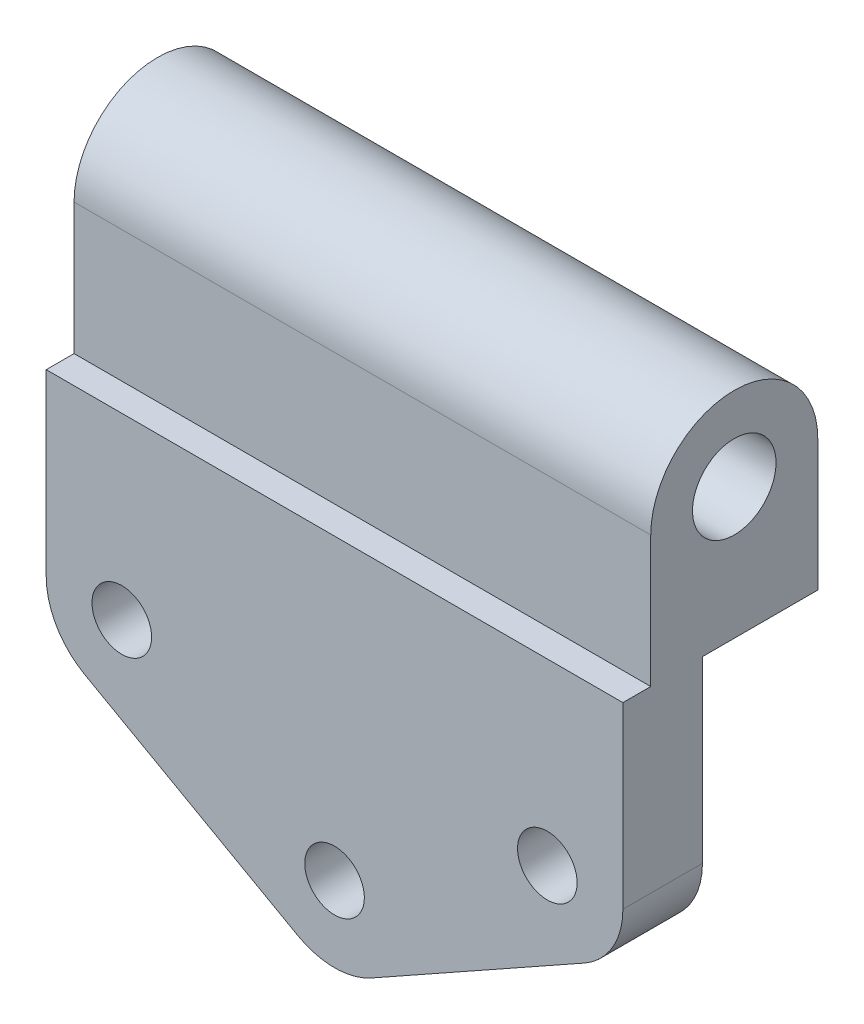
ISO-10303-21;
HEADER;
FILE_DESCRIPTION(('STEP AP214'),'2;1');
FILE_NAME('part.step','',(''),(''),'','','');
FILE_SCHEMA(('AUTOMOTIVE_DESIGN { 1 0 10303 214 1 1 1 1 }'));
ENDSEC;
DATA;
#1=APPLICATION_CONTEXT('core data for automotive mechanical design processes');
#2=APPLICATION_PROTOCOL_DEFINITION('international standard','automotive_design',2000,#1);
#3=PRODUCT_CONTEXT('',#1,'mechanical');
#4=PRODUCT('Part','Part','',(#3));
#5=PRODUCT_RELATED_PRODUCT_CATEGORY('part','',(#4));
#6=PRODUCT_DEFINITION_FORMATION('','',#4);
#7=PRODUCT_DEFINITION_CONTEXT('part definition',#1,'design');
#8=PRODUCT_DEFINITION('design','',#6,#7);
#9=PRODUCT_DEFINITION_SHAPE('','',#8);
#10=(LENGTH_UNIT() NAMED_UNIT(*) SI_UNIT(.MILLI.,.METRE.));
#11=(NAMED_UNIT(*) PLANE_ANGLE_UNIT() SI_UNIT($,.RADIAN.));
#12=(NAMED_UNIT(*) SI_UNIT($,.STERADIAN.) SOLID_ANGLE_UNIT());
#13=UNCERTAINTY_MEASURE_WITH_UNIT(LENGTH_MEASURE(1.E-05),#10,'distance_accuracy_value','');
#14=(GEOMETRIC_REPRESENTATION_CONTEXT(3) GLOBAL_UNCERTAINTY_ASSIGNED_CONTEXT((#13)) GLOBAL_UNIT_ASSIGNED_CONTEXT((#10,
#11,#12)) REPRESENTATION_CONTEXT('',''));
#15=CARTESIAN_POINT('',(0.,0.,0.));
#16=DIRECTION('',(0.,0.,1.));
#17=DIRECTION('',(1.,0.,0.));
#18=AXIS2_PLACEMENT_3D('',#15,#16,#17);
#19=CARTESIAN_POINT('',(-53.5,-16.9354535125797,20.));
#20=DIRECTION('',(0.,0.,1.));
#21=DIRECTION('',(1.,0.,0.));
#22=AXIS2_PLACEMENT_3D('',#19,#20,#21);
#23=PLANE('',#22);
#24=CARTESIAN_POINT('',(53.5,-16.9354535125797,20.));
#25=DIRECTION('',(0.,0.,1.));
#26=DIRECTION('',(1.,0.,0.));
#27=AXIS2_PLACEMENT_3D('',#24,#25,#26);
#28=CIRCLE('',#27,7.49226737139346);
#29=CARTESIAN_POINT('',(60.9922673713935,-16.9354535125797,20.));
#30=VERTEX_POINT('',#29);
#31=EDGE_CURVE('E198',#30,#30,#28,.T.);
#32=ORIENTED_EDGE('',*,*,#31,.F.);
#33=EDGE_LOOP('',(#32));
#34=FACE_BOUND('',#33,.T.);
#35=DIRECTION('',(0.,-1.,0.));
#36=VECTOR('',#35,1.);
#37=CARTESIAN_POINT('',(-72.5,28.0645464874203,20.));
#38=LINE('',#37,#36);
#39=CARTESIAN_POINT('',(-72.5,28.0645464874203,20.));
#40=VERTEX_POINT('',#39);
#41=CARTESIAN_POINT('',(-72.5,-16.9354535125796,20.));
#42=VERTEX_POINT('',#41);
#43=EDGE_CURVE('E158',#40,#42,#38,.T.);
#44=ORIENTED_EDGE('',*,*,#43,.T.);
#45=CARTESIAN_POINT('',(-53.5,-16.9354535125797,20.));
#46=DIRECTION('',(0.,0.,1.));
#47=DIRECTION('',(1.,0.,0.));
#48=AXIS2_PLACEMENT_3D('',#45,#46,#47);
#49=CIRCLE('',#48,19.);
#50=CARTESIAN_POINT('',(-62.792895002889,-33.5077829343984,20.));
#51=VERTEX_POINT('',#50);
#52=EDGE_CURVE('E97',#42,#51,#49,.T.);
#53=ORIENTED_EDGE('',*,*,#52,.T.);
#54=DIRECTION('',(0.872227864306251,-0.48909973699416,0.));
#55=VECTOR('',#54,1.);
#56=CARTESIAN_POINT('',(-62.792895002889,-33.5077829343984,20.));
#57=LINE('',#56,#55);
#58=CARTESIAN_POINT('',(-9.29289500288901,-63.5077829343984,20.));
#59=VERTEX_POINT('',#58);
#60=EDGE_CURVE('E173',#51,#59,#57,.T.);
#61=ORIENTED_EDGE('',*,*,#60,.T.);
#62=CARTESIAN_POINT('',(0.,-46.9354535125796,20.));
#63=DIRECTION('',(0.,0.,1.));
#64=DIRECTION('',(1.,0.,0.));
#65=AXIS2_PLACEMENT_3D('',#62,#63,#64);
#66=CIRCLE('',#65,19.);
#67=CARTESIAN_POINT('',(9.29289500288904,-63.5077829343984,20.));
#68=VERTEX_POINT('',#67);
#69=EDGE_CURVE('E186',#59,#68,#66,.T.);
#70=ORIENTED_EDGE('',*,*,#69,.T.);
#71=DIRECTION('',(0.872227864306251,0.489099736994159,0.));
#72=VECTOR('',#71,1.);
#73=CARTESIAN_POINT('',(62.792895002889,-33.5077829343985,20.));
#74=LINE('',#73,#72);
#75=CARTESIAN_POINT('',(62.792895002889,-33.5077829343985,20.));
#76=VERTEX_POINT('',#75);
#77=EDGE_CURVE('E117',#68,#76,#74,.T.);
#78=ORIENTED_EDGE('',*,*,#77,.T.);
#79=CARTESIAN_POINT('',(53.5,-16.9354535125797,20.));
#80=DIRECTION('',(0.,0.,1.));
#81=DIRECTION('',(1.,0.,0.));
#82=AXIS2_PLACEMENT_3D('',#79,#80,#81);
#83=CIRCLE('',#82,19.);
#84=CARTESIAN_POINT('',(72.5,-16.9354535125797,20.));
#85=VERTEX_POINT('',#84);
#86=EDGE_CURVE('E111',#76,#85,#83,.T.);
#87=ORIENTED_EDGE('',*,*,#86,.T.);
#88=DIRECTION('',(0.,1.,0.));
#89=VECTOR('',#88,1.);
#90=CARTESIAN_POINT('',(72.5,28.0645464874203,20.));
#91=LINE('',#90,#89);
#92=CARTESIAN_POINT('',(72.5,28.0645464874203,20.));
#93=VERTEX_POINT('',#92);
#94=EDGE_CURVE('E116',#85,#93,#91,.T.);
#95=ORIENTED_EDGE('',*,*,#94,.T.);
#96=DIRECTION('',(-1.,0.,0.));
#97=VECTOR('',#96,1.);
#98=CARTESIAN_POINT('',(-72.5,28.0645464874203,20.));
#99=LINE('',#98,#97);
#100=EDGE_CURVE('E65',#93,#40,#99,.T.);
#101=ORIENTED_EDGE('',*,*,#100,.T.);
#102=EDGE_LOOP('',(#44,#53,#61,#70,#78,#87,#95,#101));
#103=FACE_BOUND('',#102,.T.);
#104=CARTESIAN_POINT('',(0.,-46.9354535125796,20.));
#105=DIRECTION('',(0.,0.,1.));
#106=DIRECTION('',(1.,0.,0.));
#107=AXIS2_PLACEMENT_3D('',#104,#105,#106);
#108=CIRCLE('',#107,7.49226737139346);
#109=CARTESIAN_POINT('',(7.49226737139348,-46.9354535125796,20.));
#110=VERTEX_POINT('',#109);
#111=EDGE_CURVE('E145',#110,#110,#108,.T.);
#112=ORIENTED_EDGE('',*,*,#111,.F.);
#113=EDGE_LOOP('',(#112));
#114=FACE_BOUND('',#113,.T.);
#115=CARTESIAN_POINT('',(-53.5,-16.9354535125797,20.));
#116=DIRECTION('',(0.,0.,1.));
#117=DIRECTION('',(1.,0.,0.));
#118=AXIS2_PLACEMENT_3D('',#115,#116,#117);
#119=CIRCLE('',#118,7.49226737139346);
#120=CARTESIAN_POINT('',(-46.0077326286065,-16.9354535125797,20.));
#121=VERTEX_POINT('',#120);
#122=EDGE_CURVE('E205',#121,#121,#119,.T.);
#123=ORIENTED_EDGE('',*,*,#122,.F.);
#124=EDGE_LOOP('',(#123));
#125=FACE_BOUND('',#124,.T.);
#126=ADVANCED_FACE('F39',(#34,#103,#114,#125),#23,.T.);
#127=CARTESIAN_POINT('',(-53.5,-16.9354535125797,0.));
#128=DIRECTION('',(0.,0.,1.));
#129=DIRECTION('',(1.,0.,0.));
#130=AXIS2_PLACEMENT_3D('',#127,#128,#129);
#131=PLANE('',#130);
#132=DIRECTION('',(0.,-1.,0.));
#133=VECTOR('',#132,1.);
#134=CARTESIAN_POINT('',(-72.5,28.0645464874203,0.));
#135=LINE('',#134,#133);
#136=CARTESIAN_POINT('',(-72.5,28.0645464874203,0.));
#137=VERTEX_POINT('',#136);
#138=CARTESIAN_POINT('',(-72.5,-16.9354535125796,0.));
#139=VERTEX_POINT('',#138);
#140=EDGE_CURVE('E136',#137,#139,#135,.T.);
#141=ORIENTED_EDGE('',*,*,#140,.F.);
#142=DIRECTION('',(-1.,0.,0.));
#143=VECTOR('',#142,1.);
#144=CARTESIAN_POINT('',(-72.5,28.0645464874203,0.));
#145=LINE('',#144,#143);
#146=CARTESIAN_POINT('',(72.5,28.0645464874203,0.));
#147=VERTEX_POINT('',#146);
#148=EDGE_CURVE('E154',#147,#137,#145,.T.);
#149=ORIENTED_EDGE('',*,*,#148,.F.);
#150=DIRECTION('',(0.,1.,0.));
#151=VECTOR('',#150,1.);
#152=CARTESIAN_POINT('',(72.5,28.0645464874203,0.));
#153=LINE('',#152,#151);
#154=CARTESIAN_POINT('',(72.5,-16.9354535125797,0.));
#155=VERTEX_POINT('',#154);
#156=EDGE_CURVE('E153',#155,#147,#153,.T.);
#157=ORIENTED_EDGE('',*,*,#156,.F.);
#158=CARTESIAN_POINT('',(53.5,-16.9354535125797,0.));
#159=DIRECTION('',(0.,0.,1.));
#160=DIRECTION('',(1.,0.,0.));
#161=AXIS2_PLACEMENT_3D('',#158,#159,#160);
#162=CIRCLE('',#161,19.);
#163=CARTESIAN_POINT('',(62.792895002889,-33.5077829343985,0.));
#164=VERTEX_POINT('',#163);
#165=EDGE_CURVE('E93',#164,#155,#162,.T.);
#166=ORIENTED_EDGE('',*,*,#165,.F.);
#167=DIRECTION('',(0.872227864306251,0.489099736994159,0.));
#168=VECTOR('',#167,1.);
#169=CARTESIAN_POINT('',(62.792895002889,-33.5077829343985,0.));
#170=LINE('',#169,#168);
#171=CARTESIAN_POINT('',(9.29289500288904,-63.5077829343984,0.));
#172=VERTEX_POINT('',#171);
#173=EDGE_CURVE('E147',#172,#164,#170,.T.);
#174=ORIENTED_EDGE('',*,*,#173,.F.);
#175=CARTESIAN_POINT('',(0.,-46.9354535125796,0.));
#176=DIRECTION('',(0.,0.,1.));
#177=DIRECTION('',(1.,0.,0.));
#178=AXIS2_PLACEMENT_3D('',#175,#176,#177);
#179=CIRCLE('',#178,19.);
#180=CARTESIAN_POINT('',(-9.29289500288901,-63.5077829343984,0.));
#181=VERTEX_POINT('',#180);
#182=EDGE_CURVE('E146',#181,#172,#179,.T.);
#183=ORIENTED_EDGE('',*,*,#182,.F.);
#184=DIRECTION('',(0.872227864306251,-0.48909973699416,0.));
#185=VECTOR('',#184,1.);
#186=CARTESIAN_POINT('',(-62.792895002889,-33.5077829343984,0.));
#187=LINE('',#186,#185);
#188=CARTESIAN_POINT('',(-62.792895002889,-33.5077829343984,0.));
#189=VERTEX_POINT('',#188);
#190=EDGE_CURVE('E148',#189,#181,#187,.T.);
#191=ORIENTED_EDGE('',*,*,#190,.F.);
#192=CARTESIAN_POINT('',(-53.5,-16.9354535125797,0.));
#193=DIRECTION('',(0.,0.,1.));
#194=DIRECTION('',(1.,0.,0.));
#195=AXIS2_PLACEMENT_3D('',#192,#193,#194);
#196=CIRCLE('',#195,19.);
#197=EDGE_CURVE('E141',#139,#189,#196,.T.);
#198=ORIENTED_EDGE('',*,*,#197,.F.);
#199=EDGE_LOOP('',(#141,#149,#157,#166,#174,#183,#191,#198));
#200=FACE_BOUND('',#199,.T.);
#201=CARTESIAN_POINT('',(0.,-46.9354535125796,0.));
#202=DIRECTION('',(0.,0.,1.));
#203=DIRECTION('',(1.,0.,0.));
#204=AXIS2_PLACEMENT_3D('',#201,#202,#203);
#205=CIRCLE('',#204,7.49226737139346);
#206=CARTESIAN_POINT('',(7.49226737139348,-46.9354535125796,0.));
#207=VERTEX_POINT('',#206);
#208=EDGE_CURVE('E192',#207,#207,#205,.T.);
#209=ORIENTED_EDGE('',*,*,#208,.T.);
#210=EDGE_LOOP('',(#209));
#211=FACE_BOUND('',#210,.T.);
#212=CARTESIAN_POINT('',(53.5,-16.9354535125797,0.));
#213=DIRECTION('',(0.,0.,1.));
#214=DIRECTION('',(1.,0.,0.));
#215=AXIS2_PLACEMENT_3D('',#212,#213,#214);
#216=CIRCLE('',#215,7.49226737139346);
#217=CARTESIAN_POINT('',(60.9922673713935,-16.9354535125797,0.));
#218=VERTEX_POINT('',#217);
#219=EDGE_CURVE('E200',#218,#218,#216,.T.);
#220=ORIENTED_EDGE('',*,*,#219,.T.);
#221=EDGE_LOOP('',(#220));
#222=FACE_BOUND('',#221,.T.);
#223=CARTESIAN_POINT('',(-53.5,-16.9354535125797,0.));
#224=DIRECTION('',(0.,0.,1.));
#225=DIRECTION('',(1.,0.,0.));
#226=AXIS2_PLACEMENT_3D('',#223,#224,#225);
#227=CIRCLE('',#226,7.49226737139346);
#228=CARTESIAN_POINT('',(-46.0077326286065,-16.9354535125797,0.));
#229=VERTEX_POINT('',#228);
#230=EDGE_CURVE('E202',#229,#229,#227,.T.);
#231=ORIENTED_EDGE('',*,*,#230,.T.);
#232=EDGE_LOOP('',(#231));
#233=FACE_BOUND('',#232,.T.);
#234=ADVANCED_FACE('F177',(#200,#211,#222,#233),#131,.F.);
#235=CARTESIAN_POINT('',(-72.5,28.0645464874203,20.));
#236=DIRECTION('',(1.,0.,0.));
#237=DIRECTION('',(0.,0.,-1.));
#238=AXIS2_PLACEMENT_3D('',#235,#236,#237);
#239=PLANE('',#238);
#240=ORIENTED_EDGE('',*,*,#140,.T.);
#241=DIRECTION('',(0.,0.,-1.));
#242=VECTOR('',#241,1.);
#243=CARTESIAN_POINT('',(-72.5,-16.9354535125796,20.));
#244=LINE('',#243,#242);
#245=EDGE_CURVE('E11',#42,#139,#244,.T.);
#246=ORIENTED_EDGE('',*,*,#245,.F.);
#247=ORIENTED_EDGE('',*,*,#43,.F.);
#248=DIRECTION('',(0.,0.,-1.));
#249=VECTOR('',#248,1.);
#250=CARTESIAN_POINT('',(-72.5,28.0645464874203,20.));
#251=LINE('',#250,#249);
#252=CARTESIAN_POINT('',(-72.5,28.0645464874203,13.));
#253=VERTEX_POINT('',#252);
#254=EDGE_CURVE('E138',#40,#253,#251,.T.);
#255=ORIENTED_EDGE('',*,*,#254,.T.);
#256=DIRECTION('',(0.,-1.,0.));
#257=VECTOR('',#256,1.);
#258=CARTESIAN_POINT('',(-72.5,61.0645464874204,13.));
#259=LINE('',#258,#257);
#260=CARTESIAN_POINT('',(-72.5,61.0645464874204,13.));
#261=VERTEX_POINT('',#260);
#262=EDGE_CURVE('E53',#261,#253,#259,.T.);
#263=ORIENTED_EDGE('',*,*,#262,.F.);
#264=CARTESIAN_POINT('',(-72.5,61.0645464874203,-8.));
#265=DIRECTION('',(1.,0.,0.));
#266=DIRECTION('',(0.,0.,-1.));
#267=AXIS2_PLACEMENT_3D('',#264,#265,#266);
#268=CIRCLE('',#267,21.);
#269=CARTESIAN_POINT('',(-72.5,61.0645464874204,-29.));
#270=VERTEX_POINT('',#269);
#271=EDGE_CURVE('E228',#270,#261,#268,.T.);
#272=ORIENTED_EDGE('',*,*,#271,.F.);
#273=DIRECTION('',(0.,1.,0.));
#274=VECTOR('',#273,1.);
#275=CARTESIAN_POINT('',(-72.5,61.0645464874204,-29.));
#276=LINE('',#275,#274);
#277=CARTESIAN_POINT('',(-72.5,28.0645464874203,-29.));
#278=VERTEX_POINT('',#277);
#279=EDGE_CURVE('E222',#278,#270,#276,.T.);
#280=ORIENTED_EDGE('',*,*,#279,.F.);
#281=DIRECTION('',(0.,0.,-1.));
#282=VECTOR('',#281,1.);
#283=CARTESIAN_POINT('',(-72.5,28.0645464874203,13.));
#284=LINE('',#283,#282);
#285=EDGE_CURVE('E223',#137,#278,#284,.T.);
#286=ORIENTED_EDGE('',*,*,#285,.F.);
#287=EDGE_LOOP('',(#240,#246,#247,#255,#263,#272,#280,#286));
#288=FACE_BOUND('',#287,.T.);
#289=CARTESIAN_POINT('',(-72.5,61.0645464874203,-8.));
#290=DIRECTION('',(1.,0.,0.));
#291=DIRECTION('',(0.,0.,-1.));
#292=AXIS2_PLACEMENT_3D('',#289,#290,#291);
#293=CIRCLE('',#292,10.5);
#294=CARTESIAN_POINT('',(-72.5,61.0645464874203,-18.5));
#295=VERTEX_POINT('',#294);
#296=EDGE_CURVE('E241',#295,#295,#293,.T.);
#297=ORIENTED_EDGE('',*,*,#296,.T.);
#298=EDGE_LOOP('',(#297));
#299=FACE_BOUND('',#298,.T.);
#300=ADVANCED_FACE('F41',(#288,#299),#239,.F.);
#301=CARTESIAN_POINT('',(-53.5,-16.9354535125797,20.));
#302=DIRECTION('',(0.,0.,-1.));
#303=DIRECTION('',(-1.,0.,0.));
#304=AXIS2_PLACEMENT_3D('',#301,#302,#303);
#305=CYLINDRICAL_SURFACE('',#304,19.);
#306=ORIENTED_EDGE('',*,*,#197,.T.);
#307=DIRECTION('',(0.,0.,-1.));
#308=VECTOR('',#307,1.);
#309=CARTESIAN_POINT('',(-62.792895002889,-33.5077829343984,20.));
#310=LINE('',#309,#308);
#311=EDGE_CURVE('E50',#51,#189,#310,.T.);
#312=ORIENTED_EDGE('',*,*,#311,.F.);
#313=ORIENTED_EDGE('',*,*,#52,.F.);
#314=ORIENTED_EDGE('',*,*,#245,.T.);
#315=EDGE_LOOP('',(#306,#312,#313,#314));
#316=FACE_BOUND('',#315,.T.);
#317=ADVANCED_FACE('F359',(#316),#305,.T.);
#318=CARTESIAN_POINT('',(-62.792895002889,-33.5077829343984,20.));
#319=DIRECTION('',(0.48909973699416,0.872227864306251,0.));
#320=DIRECTION('',(-0.872227864306251,0.48909973699416,0.));
#321=AXIS2_PLACEMENT_3D('',#318,#319,#320);
#322=PLANE('',#321);
#323=ORIENTED_EDGE('',*,*,#190,.T.);
#324=DIRECTION('',(0.,0.,-1.));
#325=VECTOR('',#324,1.);
#326=CARTESIAN_POINT('',(-9.29289500288901,-63.5077829343984,20.));
#327=LINE('',#326,#325);
#328=EDGE_CURVE('E167',#59,#181,#327,.T.);
#329=ORIENTED_EDGE('',*,*,#328,.F.);
#330=ORIENTED_EDGE('',*,*,#60,.F.);
#331=ORIENTED_EDGE('',*,*,#311,.T.);
#332=EDGE_LOOP('',(#323,#329,#330,#331));
#333=FACE_BOUND('',#332,.T.);
#334=ADVANCED_FACE('F171',(#333),#322,.F.);
#335=CARTESIAN_POINT('',(0.,-46.9354535125796,20.));
#336=DIRECTION('',(0.,0.,-1.));
#337=DIRECTION('',(-1.,0.,0.));
#338=AXIS2_PLACEMENT_3D('',#335,#336,#337);
#339=CYLINDRICAL_SURFACE('',#338,19.);
#340=ORIENTED_EDGE('',*,*,#182,.T.);
#341=DIRECTION('',(0.,0.,-1.));
#342=VECTOR('',#341,1.);
#343=CARTESIAN_POINT('',(9.29289500288904,-63.5077829343984,20.));
#344=LINE('',#343,#342);
#345=EDGE_CURVE('E162',#68,#172,#344,.T.);
#346=ORIENTED_EDGE('',*,*,#345,.F.);
#347=ORIENTED_EDGE('',*,*,#69,.F.);
#348=ORIENTED_EDGE('',*,*,#328,.T.);
#349=EDGE_LOOP('',(#340,#346,#347,#348));
#350=FACE_BOUND('',#349,.T.);
#351=ADVANCED_FACE('F181',(#350),#339,.T.);
#352=CARTESIAN_POINT('',(62.792895002889,-33.5077829343985,20.));
#353=DIRECTION('',(-0.489099736994159,0.872227864306251,0.));
#354=DIRECTION('',(-0.872227864306251,-0.489099736994159,0.));
#355=AXIS2_PLACEMENT_3D('',#352,#353,#354);
#356=PLANE('',#355);
#357=ORIENTED_EDGE('',*,*,#173,.T.);
#358=DIRECTION('',(0.,0.,-1.));
#359=VECTOR('',#358,1.);
#360=CARTESIAN_POINT('',(62.792895002889,-33.5077829343985,20.));
#361=LINE('',#360,#359);
#362=EDGE_CURVE('E126',#76,#164,#361,.T.);
#363=ORIENTED_EDGE('',*,*,#362,.F.);
#364=ORIENTED_EDGE('',*,*,#77,.F.);
#365=ORIENTED_EDGE('',*,*,#345,.T.);
#366=EDGE_LOOP('',(#357,#363,#364,#365));
#367=FACE_BOUND('',#366,.T.);
#368=ADVANCED_FACE('F189',(#367),#356,.F.);
#369=CARTESIAN_POINT('',(53.5,-16.9354535125797,20.));
#370=DIRECTION('',(0.,0.,-1.));
#371=DIRECTION('',(-1.,0.,0.));
#372=AXIS2_PLACEMENT_3D('',#369,#370,#371);
#373=CYLINDRICAL_SURFACE('',#372,19.);
#374=ORIENTED_EDGE('',*,*,#165,.T.);
#375=DIRECTION('',(0.,0.,-1.));
#376=VECTOR('',#375,1.);
#377=CARTESIAN_POINT('',(72.5,-16.9354535125797,20.));
#378=LINE('',#377,#376);
#379=EDGE_CURVE('E122',#85,#155,#378,.T.);
#380=ORIENTED_EDGE('',*,*,#379,.F.);
#381=ORIENTED_EDGE('',*,*,#86,.F.);
#382=ORIENTED_EDGE('',*,*,#362,.T.);
#383=EDGE_LOOP('',(#374,#380,#381,#382));
#384=FACE_BOUND('',#383,.T.);
#385=ADVANCED_FACE('F125',(#384),#373,.T.);
#386=CARTESIAN_POINT('',(72.5,28.0645464874203,20.));
#387=DIRECTION('',(-1.,0.,0.));
#388=DIRECTION('',(0.,-1.,0.));
#389=AXIS2_PLACEMENT_3D('',#386,#387,#388);
#390=PLANE('',#389);
#391=ORIENTED_EDGE('',*,*,#156,.T.);
#392=DIRECTION('',(0.,0.,-1.));
#393=VECTOR('',#392,1.);
#394=CARTESIAN_POINT('',(72.5,28.0645464874203,13.));
#395=LINE('',#394,#393);
#396=CARTESIAN_POINT('',(72.5,28.0645464874203,-29.));
#397=VERTEX_POINT('',#396);
#398=EDGE_CURVE('E231',#147,#397,#395,.T.);
#399=ORIENTED_EDGE('',*,*,#398,.T.);
#400=DIRECTION('',(0.,1.,0.));
#401=VECTOR('',#400,1.);
#402=CARTESIAN_POINT('',(72.5,61.0645464874204,-29.));
#403=LINE('',#402,#401);
#404=CARTESIAN_POINT('',(72.5,61.0645464874204,-29.));
#405=VERTEX_POINT('',#404);
#406=EDGE_CURVE('E219',#397,#405,#403,.T.);
#407=ORIENTED_EDGE('',*,*,#406,.T.);
#408=CARTESIAN_POINT('',(72.5,61.0645464874203,-8.));
#409=DIRECTION('',(1.,0.,0.));
#410=DIRECTION('',(0.,0.,-1.));
#411=AXIS2_PLACEMENT_3D('',#408,#409,#410);
#412=CIRCLE('',#411,21.);
#413=CARTESIAN_POINT('',(72.5,61.0645464874204,13.));
#414=VERTEX_POINT('',#413);
#415=EDGE_CURVE('E221',#405,#414,#412,.T.);
#416=ORIENTED_EDGE('',*,*,#415,.T.);
#417=DIRECTION('',(0.,-1.,0.));
#418=VECTOR('',#417,1.);
#419=CARTESIAN_POINT('',(72.5,61.0645464874204,13.));
#420=LINE('',#419,#418);
#421=CARTESIAN_POINT('',(72.5,28.0645464874203,13.));
#422=VERTEX_POINT('',#421);
#423=EDGE_CURVE('E236',#414,#422,#420,.T.);
#424=ORIENTED_EDGE('',*,*,#423,.T.);
#425=DIRECTION('',(0.,0.,-1.));
#426=VECTOR('',#425,1.);
#427=CARTESIAN_POINT('',(72.5,28.0645464874203,20.));
#428=LINE('',#427,#426);
#429=EDGE_CURVE('E129',#93,#422,#428,.T.);
#430=ORIENTED_EDGE('',*,*,#429,.F.);
#431=ORIENTED_EDGE('',*,*,#94,.F.);
#432=ORIENTED_EDGE('',*,*,#379,.T.);
#433=EDGE_LOOP('',(#391,#399,#407,#416,#424,#430,#431,#432));
#434=FACE_BOUND('',#433,.T.);
#435=CARTESIAN_POINT('',(72.5,61.0645464874203,-8.));
#436=DIRECTION('',(1.,0.,0.));
#437=DIRECTION('',(0.,0.,-1.));
#438=AXIS2_PLACEMENT_3D('',#435,#436,#437);
#439=CIRCLE('',#438,10.5);
#440=CARTESIAN_POINT('',(72.5,61.0645464874203,-18.5));
#441=VERTEX_POINT('',#440);
#442=EDGE_CURVE('E234',#441,#441,#439,.T.);
#443=ORIENTED_EDGE('',*,*,#442,.F.);
#444=EDGE_LOOP('',(#443));
#445=FACE_BOUND('',#444,.T.);
#446=ADVANCED_FACE('F134',(#434,#445),#390,.F.);
#447=CARTESIAN_POINT('',(-72.5,28.0645464874203,20.));
#448=DIRECTION('',(0.,-1.,0.));
#449=DIRECTION('',(0.,0.,-1.));
#450=AXIS2_PLACEMENT_3D('',#447,#448,#449);
#451=PLANE('',#450);
#452=ORIENTED_EDGE('',*,*,#429,.T.);
#453=DIRECTION('',(-1.,0.,0.));
#454=VECTOR('',#453,1.);
#455=CARTESIAN_POINT('',(72.5,28.0645464874203,13.));
#456=LINE('',#455,#454);
#457=EDGE_CURVE('E215',#422,#253,#456,.T.);
#458=ORIENTED_EDGE('',*,*,#457,.T.);
#459=ORIENTED_EDGE('',*,*,#254,.F.);
#460=ORIENTED_EDGE('',*,*,#100,.F.);
#461=EDGE_LOOP('',(#452,#458,#459,#460));
#462=FACE_BOUND('',#461,.T.);
#463=ADVANCED_FACE('F253',(#462),#451,.F.);
#464=CARTESIAN_POINT('',(0.,-46.9354535125796,20.));
#465=DIRECTION('',(0.,0.,-1.));
#466=DIRECTION('',(-1.,0.,0.));
#467=AXIS2_PLACEMENT_3D('',#464,#465,#466);
#468=CYLINDRICAL_SURFACE('',#467,7.49226737139346);
#469=ORIENTED_EDGE('',*,*,#111,.T.);
#470=EDGE_LOOP('',(#469));
#471=FACE_BOUND('',#470,.T.);
#472=ORIENTED_EDGE('',*,*,#208,.F.);
#473=EDGE_LOOP('',(#472));
#474=FACE_BOUND('',#473,.T.);
#475=ADVANCED_FACE('F260',(#471,#474),#468,.F.);
#476=CARTESIAN_POINT('',(53.5,-16.9354535125797,20.));
#477=DIRECTION('',(0.,0.,-1.));
#478=DIRECTION('',(-1.,0.,0.));
#479=AXIS2_PLACEMENT_3D('',#476,#477,#478);
#480=CYLINDRICAL_SURFACE('',#479,7.49226737139346);
#481=ORIENTED_EDGE('',*,*,#31,.T.);
#482=EDGE_LOOP('',(#481));
#483=FACE_BOUND('',#482,.T.);
#484=ORIENTED_EDGE('',*,*,#219,.F.);
#485=EDGE_LOOP('',(#484));
#486=FACE_BOUND('',#485,.T.);
#487=ADVANCED_FACE('F273',(#483,#486),#480,.F.);
#488=CARTESIAN_POINT('',(-53.5,-16.9354535125797,20.));
#489=DIRECTION('',(0.,0.,-1.));
#490=DIRECTION('',(-1.,0.,0.));
#491=AXIS2_PLACEMENT_3D('',#488,#489,#490);
#492=CYLINDRICAL_SURFACE('',#491,7.49226737139346);
#493=ORIENTED_EDGE('',*,*,#122,.T.);
#494=EDGE_LOOP('',(#493));
#495=FACE_BOUND('',#494,.T.);
#496=ORIENTED_EDGE('',*,*,#230,.F.);
#497=EDGE_LOOP('',(#496));
#498=FACE_BOUND('',#497,.T.);
#499=ADVANCED_FACE('F279',(#495,#498),#492,.F.);
#500=CARTESIAN_POINT('',(72.5,28.0645464874203,13.));
#501=DIRECTION('',(0.,1.,0.));
#502=DIRECTION('',(0.,0.,1.));
#503=AXIS2_PLACEMENT_3D('',#500,#501,#502);
#504=PLANE('',#503);
#505=ORIENTED_EDGE('',*,*,#398,.F.);
#506=ORIENTED_EDGE('',*,*,#148,.T.);
#507=ORIENTED_EDGE('',*,*,#285,.T.);
#508=DIRECTION('',(-1.,0.,0.));
#509=VECTOR('',#508,1.);
#510=CARTESIAN_POINT('',(72.5,28.0645464874203,-29.));
#511=LINE('',#510,#509);
#512=EDGE_CURVE('E212',#397,#278,#511,.T.);
#513=ORIENTED_EDGE('',*,*,#512,.F.);
#514=EDGE_LOOP('',(#505,#506,#507,#513));
#515=FACE_BOUND('',#514,.T.);
#516=ADVANCED_FACE('F281',(#515),#504,.F.);
#517=CARTESIAN_POINT('',(72.5,61.0645464874203,-8.));
#518=DIRECTION('',(-1.,0.,0.));
#519=DIRECTION('',(0.,0.,1.));
#520=AXIS2_PLACEMENT_3D('',#517,#518,#519);
#521=CYLINDRICAL_SURFACE('',#520,21.);
#522=ORIENTED_EDGE('',*,*,#271,.T.);
#523=DIRECTION('',(-1.,0.,0.));
#524=VECTOR('',#523,1.);
#525=CARTESIAN_POINT('',(72.5,61.0645464874204,13.));
#526=LINE('',#525,#524);
#527=EDGE_CURVE('E208',#414,#261,#526,.T.);
#528=ORIENTED_EDGE('',*,*,#527,.F.);
#529=ORIENTED_EDGE('',*,*,#415,.F.);
#530=DIRECTION('',(-1.,0.,0.));
#531=VECTOR('',#530,1.);
#532=CARTESIAN_POINT('',(72.5,61.0645464874204,-29.));
#533=LINE('',#532,#531);
#534=EDGE_CURVE('E220',#405,#270,#533,.T.);
#535=ORIENTED_EDGE('',*,*,#534,.T.);
#536=EDGE_LOOP('',(#522,#528,#529,#535));
#537=FACE_BOUND('',#536,.T.);
#538=ADVANCED_FACE('F283',(#537),#521,.T.);
#539=CARTESIAN_POINT('',(72.5,61.0645464874204,13.));
#540=DIRECTION('',(0.,0.,-1.));
#541=DIRECTION('',(-1.,0.,0.));
#542=AXIS2_PLACEMENT_3D('',#539,#540,#541);
#543=PLANE('',#542);
#544=ORIENTED_EDGE('',*,*,#262,.T.);
#545=ORIENTED_EDGE('',*,*,#457,.F.);
#546=ORIENTED_EDGE('',*,*,#423,.F.);
#547=ORIENTED_EDGE('',*,*,#527,.T.);
#548=EDGE_LOOP('',(#544,#545,#546,#547));
#549=FACE_BOUND('',#548,.T.);
#550=ADVANCED_FACE('F289',(#549),#543,.F.);
#551=CARTESIAN_POINT('',(72.5,61.0645464874204,-29.));
#552=DIRECTION('',(0.,0.,1.));
#553=DIRECTION('',(1.,0.,0.));
#554=AXIS2_PLACEMENT_3D('',#551,#552,#553);
#555=PLANE('',#554);
#556=ORIENTED_EDGE('',*,*,#279,.T.);
#557=ORIENTED_EDGE('',*,*,#534,.F.);
#558=ORIENTED_EDGE('',*,*,#406,.F.);
#559=ORIENTED_EDGE('',*,*,#512,.T.);
#560=EDGE_LOOP('',(#556,#557,#558,#559));
#561=FACE_BOUND('',#560,.T.);
#562=ADVANCED_FACE('F292',(#561),#555,.F.);
#563=CARTESIAN_POINT('',(72.5,61.0645464874203,-8.));
#564=DIRECTION('',(-1.,0.,0.));
#565=DIRECTION('',(0.,0.,1.));
#566=AXIS2_PLACEMENT_3D('',#563,#564,#565);
#567=CYLINDRICAL_SURFACE('',#566,10.5);
#568=ORIENTED_EDGE('',*,*,#442,.T.);
#569=EDGE_LOOP('',(#568));
#570=FACE_BOUND('',#569,.T.);
#571=ORIENTED_EDGE('',*,*,#296,.F.);
#572=EDGE_LOOP('',(#571));
#573=FACE_BOUND('',#572,.T.);
#574=ADVANCED_FACE('F247',(#570,#573),#567,.F.);
#575=CLOSED_SHELL('',(#126,#234,#300,#317,#334,#351,#368,#385,#446,#463,#475,#487,#499,#516,
#538,#550,#562,#574));
#576=MANIFOLD_SOLID_BREP('B2',#575);
#577=ADVANCED_BREP_SHAPE_REPRESENTATION('',(#18,#576),#14);
#578=SHAPE_DEFINITION_REPRESENTATION(#9,#577);
ENDSEC;
END-ISO-10303-21;
